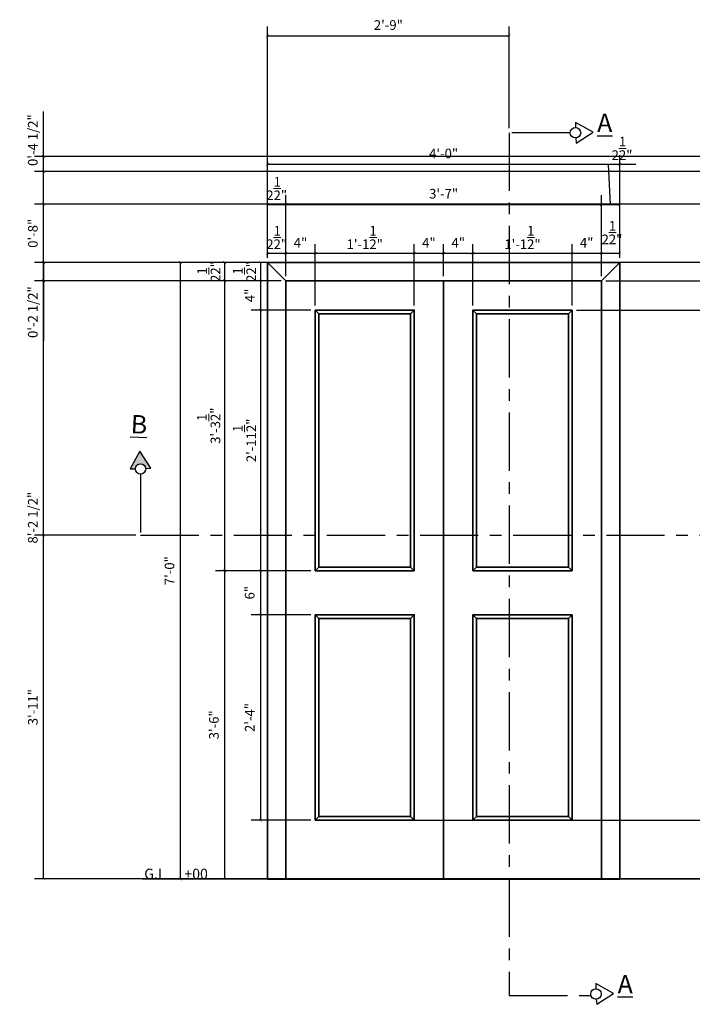
# Model space of a CAD drawing. Units: inches. Extents: x 1926 to 2169, y 1541 to 1783.
# Tile 2 of 3: x 1933 to 2025, y 1649 to 1783. Entities that reach past the tile are written whole.
import ezdxf

# ---------------------------------------------------------------- set-up
doc = ezdxf.new("R2010")
doc.units = ezdxf.units.IN
doc.linetypes.add('CENTER', pattern=[50.8, 31.75, -6.35, 6.35, -6.35])
for name, color, linetype, lineweight in [('A-ANNO-DIMS', 2, 'Continuous', 18), ('A-ANNO-SECT', 1, 'CENTER', 25), ('A-ANNO-SYMB', 1, 'Continuous', 25), ('A-DOOR', 4, 'Continuous', 35)]:
    doc.layers.add(name, color=color, linetype=linetype, lineweight=lineweight)
doc.styles.get("Standard").update_dxf_attribs({"font": 'arial.ttf'})
doc.dimstyles.new('ISO-25', dxfattribs={"dimtxt": 1.3125, "dimasz": 0.375, "dimexe": 1.25, "dimexo": 0.625, "dimtad": 1, "dimzin": 3, "dimlunit": 4, "dimtxsty": 'Standard', "dimblk": 'ARCHTICK', "dimcen": 0.09, "dimadec": 0, "dimazin": 0, "dimtfac": 1, "dimtofl": 0, "dimtmove": 0, "dimatfit": 3, "dimfxl": 1, "dimarcsym": 0})
pattern_1 = [(0, (0, 0), (0, 6.985), [5.08, -1.905]), (90, (0, 0), (-6.985, 4e-16), [5.08, -1.905])]

# ---------------------------------------------------------------- blocks, each defined once
blk = doc.blocks.new('_ArchTick')
at = {"color": 0, "linetype": 'ByBlock', "const_width": 0.15}
blk.add_lwpolyline([(-0.5, -0.5), (0.5, 0.5)], dxfattribs=at)
blk = doc.blocks.new('*D7')
at = {"layer": 'A-ANNO-DIMS', "color": 0, "lineweight": -2, "transparency": 16777216}
for p, q in [((1967.28, 1750.43), (1967.28, 1752.29)), ((1969.78, 1747.93), (1969.78, 1752.29)), ((1967.28, 1751.04), (1969.78, 1751.04))]:
    blk.add_line(p, q, dxfattribs=at)
at = {"layer": 'DEFPOINTS', "color": 0, "transparency": 16777216}
for p in [(1969.78, 1751.04), (1967.28, 1749.81), (1969.78, 1747.31)]:
    blk.add_point(p, dxfattribs=at)
at = {"layer": 'A-ANNO-DIMS', "color": 0, "lineweight": -2, "transparency": 16777216, "xscale": 0.375, "yscale": 0.375, "zscale": 0.375, "rotation": 180}
blk.add_blockref('_ArchTick', (1967.28, 1751.04), dxfattribs=at)
at = {"layer": 'A-ANNO-DIMS', "color": 0, "lineweight": -2, "transparency": 16777216, "xscale": 0.375, "yscale": 0.375, "zscale": 0.375}
blk.add_blockref('_ArchTick', (1969.78, 1751.04), dxfattribs=at)
at = {"layer": 'A-ANNO-DIMS', "color": 0, "transparency": 16777216, "insert": (1968.53, 1753.2), "char_height": 1.3125, "attachment_point": 5}
blk.add_mtext('2{\\H1x;\\S1/2;}"', dxfattribs=at)
blk = doc.blocks.new('*D8')
at = {"layer": 'A-ANNO-DIMS', "color": 0, "lineweight": -2, "transparency": 16777216}
for p, q in [((1969.78, 1747.93), (1969.78, 1752.29)), ((1973.78, 1743.93), (1973.78, 1752.29)), ((1969.78, 1751.04), (1973.78, 1751.04))]:
    blk.add_line(p, q, dxfattribs=at)
at = {"layer": 'DEFPOINTS', "color": 0, "transparency": 16777216}
for p in [(1973.78, 1751.04), (1969.78, 1747.31), (1973.78, 1743.31)]:
    blk.add_point(p, dxfattribs=at)
at = {"layer": 'A-ANNO-DIMS', "color": 0, "lineweight": -2, "transparency": 16777216, "xscale": 0.375, "yscale": 0.375, "zscale": 0.375, "rotation": 180}
blk.add_blockref('_ArchTick', (1969.78, 1751.04), dxfattribs=at)
at = {"layer": 'A-ANNO-DIMS', "color": 0, "lineweight": -2, "transparency": 16777216, "xscale": 0.375, "yscale": 0.375, "zscale": 0.375}
blk.add_blockref('_ArchTick', (1973.78, 1751.04), dxfattribs=at)
at = {"layer": 'A-ANNO-DIMS', "color": 0, "transparency": 16777216, "insert": (1971.78, 1752.32), "char_height": 1.312, "attachment_point": 5}
blk.add_mtext('4"', dxfattribs=at)
blk = doc.blocks.new('*D9')
at = {"layer": 'A-ANNO-DIMS', "color": 0, "lineweight": -2, "transparency": 16777216}
for p, q in [((1973.78, 1743.93), (1973.78, 1752.29)), ((1987.28, 1743.93), (1987.28, 1752.29)), ((1973.78, 1751.04), (1987.28, 1751.04))]:
    blk.add_line(p, q, dxfattribs=at)
at = {"layer": 'DEFPOINTS', "color": 0, "transparency": 16777216}
for p in [(1987.28, 1751.04), (1973.78, 1743.31), (1987.28, 1743.31)]:
    blk.add_point(p, dxfattribs=at)
at = {"layer": 'A-ANNO-DIMS', "color": 0, "lineweight": -2, "transparency": 16777216, "xscale": 0.375, "yscale": 0.375, "zscale": 0.375, "rotation": 180}
blk.add_blockref('_ArchTick', (1973.78, 1751.04), dxfattribs=at)
at = {"layer": 'A-ANNO-DIMS', "color": 0, "lineweight": -2, "transparency": 16777216, "xscale": 0.375, "yscale": 0.375, "zscale": 0.375}
blk.add_blockref('_ArchTick', (1987.28, 1751.04), dxfattribs=at)
at = {"layer": 'A-ANNO-DIMS', "color": 0, "transparency": 16777216, "insert": (1980.53, 1753.2), "char_height": 1.3125, "attachment_point": 5}
blk.add_mtext('1\'-1{\\H1x;\\S1/2;}"', dxfattribs=at)
blk = doc.blocks.new('*D10')
at = {"layer": 'A-ANNO-DIMS', "color": 0, "lineweight": -2, "transparency": 16777216}
for p, q in [((1987.28, 1743.93), (1987.28, 1752.29)), ((1991.28, 1747.93), (1991.28, 1752.29)), ((1987.28, 1751.04), (1991.28, 1751.04))]:
    blk.add_line(p, q, dxfattribs=at)
at = {"layer": 'DEFPOINTS', "color": 0, "transparency": 16777216}
for p in [(1991.28, 1751.04), (1991.28, 1747.31), (1987.28, 1743.31)]:
    blk.add_point(p, dxfattribs=at)
at = {"layer": 'A-ANNO-DIMS', "color": 0, "lineweight": -2, "transparency": 16777216, "xscale": 0.375, "yscale": 0.375, "zscale": 0.375, "rotation": 180}
blk.add_blockref('_ArchTick', (1987.28, 1751.04), dxfattribs=at)
at = {"layer": 'A-ANNO-DIMS', "color": 0, "lineweight": -2, "transparency": 16777216, "xscale": 0.375, "yscale": 0.375, "zscale": 0.375}
blk.add_blockref('_ArchTick', (1991.28, 1751.04), dxfattribs=at)
at = {"layer": 'A-ANNO-DIMS', "color": 0, "transparency": 16777216, "insert": (1989.28, 1752.32), "char_height": 1.312, "attachment_point": 5}
blk.add_mtext('4"', dxfattribs=at)
blk = doc.blocks.new('*D11')
at = {"layer": 'A-ANNO-DIMS', "color": 0, "lineweight": -2, "transparency": 16777216}
for p, q in [((1991.28, 1747.93), (1991.28, 1752.29)), ((1995.28, 1743.93), (1995.28, 1752.29)), ((1991.28, 1751.04), (1995.28, 1751.04))]:
    blk.add_line(p, q, dxfattribs=at)
at = {"layer": 'DEFPOINTS', "color": 0, "transparency": 16777216}
for p in [(1995.28, 1751.04), (1991.28, 1747.31), (1995.28, 1743.31)]:
    blk.add_point(p, dxfattribs=at)
at = {"layer": 'A-ANNO-DIMS', "color": 0, "lineweight": -2, "transparency": 16777216, "xscale": 0.375, "yscale": 0.375, "zscale": 0.375, "rotation": 180}
blk.add_blockref('_ArchTick', (1991.28, 1751.04), dxfattribs=at)
at = {"layer": 'A-ANNO-DIMS', "color": 0, "lineweight": -2, "transparency": 16777216, "xscale": 0.375, "yscale": 0.375, "zscale": 0.375}
blk.add_blockref('_ArchTick', (1995.28, 1751.04), dxfattribs=at)
at = {"layer": 'A-ANNO-DIMS', "color": 0, "transparency": 16777216, "insert": (1993.28, 1752.32), "char_height": 1.312, "attachment_point": 5}
blk.add_mtext('4"', dxfattribs=at)
blk = doc.blocks.new('*D12')
at = {"layer": 'A-ANNO-DIMS', "color": 0, "lineweight": -2, "transparency": 16777216}
for p, q in [((1995.28, 1743.93), (1995.28, 1752.29)), ((2008.78, 1743.93), (2008.78, 1752.29)), ((1995.28, 1751.04), (2008.78, 1751.04))]:
    blk.add_line(p, q, dxfattribs=at)
at = {"layer": 'DEFPOINTS', "color": 0, "transparency": 16777216}
for p in [(2008.78, 1751.04), (1995.28, 1743.31), (2008.78, 1743.31)]:
    blk.add_point(p, dxfattribs=at)
at = {"layer": 'A-ANNO-DIMS', "color": 0, "lineweight": -2, "transparency": 16777216, "xscale": 0.375, "yscale": 0.375, "zscale": 0.375, "rotation": 180}
blk.add_blockref('_ArchTick', (1995.28, 1751.04), dxfattribs=at)
at = {"layer": 'A-ANNO-DIMS', "color": 0, "lineweight": -2, "transparency": 16777216, "xscale": 0.375, "yscale": 0.375, "zscale": 0.375}
blk.add_blockref('_ArchTick', (2008.78, 1751.04), dxfattribs=at)
at = {"layer": 'A-ANNO-DIMS', "color": 0, "transparency": 16777216, "insert": (2002.03, 1753.2), "char_height": 1.3125, "attachment_point": 5}
blk.add_mtext('1\'-1{\\H1x;\\S1/2;}"', dxfattribs=at)
blk = doc.blocks.new('*D13')
at = {"layer": 'A-ANNO-DIMS', "color": 0, "lineweight": -2, "transparency": 16777216}
for p, q in [((2008.78, 1743.93), (2008.78, 1752.29)), ((2012.78, 1747.93), (2012.78, 1752.29)), ((2008.78, 1751.04), (2012.78, 1751.04))]:
    blk.add_line(p, q, dxfattribs=at)
at = {"layer": 'DEFPOINTS', "color": 0, "transparency": 16777216}
for p in [(2012.78, 1751.04), (2012.78, 1747.31), (2008.78, 1743.31)]:
    blk.add_point(p, dxfattribs=at)
at = {"layer": 'A-ANNO-DIMS', "color": 0, "lineweight": -2, "transparency": 16777216, "xscale": 0.375, "yscale": 0.375, "zscale": 0.375, "rotation": 180}
blk.add_blockref('_ArchTick', (2008.78, 1751.04), dxfattribs=at)
at = {"layer": 'A-ANNO-DIMS', "color": 0, "lineweight": -2, "transparency": 16777216, "xscale": 0.375, "yscale": 0.375, "zscale": 0.375}
blk.add_blockref('_ArchTick', (2012.78, 1751.04), dxfattribs=at)
at = {"layer": 'A-ANNO-DIMS', "color": 0, "transparency": 16777216, "insert": (2010.78, 1752.32), "char_height": 1.312, "attachment_point": 5}
blk.add_mtext('4"', dxfattribs=at)
blk = doc.blocks.new('*D14')
at = {"layer": 'A-ANNO-DIMS', "color": 0, "lineweight": -2, "transparency": 16777216}
for p, q in [((2012.78, 1747.93), (2012.78, 1752.29)), ((2015.28, 1750.43), (2015.28, 1752.29)), ((2012.78, 1751.04), (2015.28, 1751.04))]:
    blk.add_line(p, q, dxfattribs=at)
at = {"layer": 'DEFPOINTS', "color": 0, "transparency": 16777216}
for p in [(2015.28, 1751.04), (2015.28, 1749.81), (2012.78, 1747.31)]:
    blk.add_point(p, dxfattribs=at)
at = {"layer": 'A-ANNO-DIMS', "color": 0, "lineweight": -2, "transparency": 16777216, "xscale": 0.375, "yscale": 0.375, "zscale": 0.375, "rotation": 180}
blk.add_blockref('_ArchTick', (2012.78, 1751.04), dxfattribs=at)
at = {"layer": 'A-ANNO-DIMS', "color": 0, "lineweight": -2, "transparency": 16777216, "xscale": 0.375, "yscale": 0.375, "zscale": 0.375}
blk.add_blockref('_ArchTick', (2015.28, 1751.04), dxfattribs=at)
at = {"layer": 'A-ANNO-DIMS', "color": 0, "transparency": 16777216, "insert": (2014.23, 1753.86), "char_height": 1.3125, "attachment_point": 5}
blk.add_mtext('2{\\H1x;\\S1/2;}"', dxfattribs=at)
blk = doc.blocks.new('*D15')
at = {"layer": 'A-ANNO-DIMS', "color": 0, "lineweight": -2, "transparency": 16777216}
for p, q in [((1967.28, 1750.43), (1967.28, 1764.43)), ((2015.28, 1750.43), (2015.28, 1764.43)), ((1967.28, 1763.18), (2015.28, 1763.18))]:
    blk.add_line(p, q, dxfattribs=at)
at = {"layer": 'DEFPOINTS', "color": 0, "transparency": 16777216}
for p in [(2015.28, 1763.18), (1967.28, 1749.81), (2015.28, 1749.81)]:
    blk.add_point(p, dxfattribs=at)
at = {"layer": 'A-ANNO-DIMS', "color": 0, "lineweight": -2, "transparency": 16777216, "xscale": 0.375, "yscale": 0.375, "zscale": 0.375, "rotation": 180}
blk.add_blockref('_ArchTick', (1967.28, 1763.18), dxfattribs=at)
at = {"layer": 'A-ANNO-DIMS', "color": 0, "lineweight": -2, "transparency": 16777216, "xscale": 0.375, "yscale": 0.375, "zscale": 0.375}
blk.add_blockref('_ArchTick', (2015.28, 1763.18), dxfattribs=at)
at = {"layer": 'A-ANNO-DIMS', "color": 0, "transparency": 16777216, "insert": (1991.28, 1764.47), "char_height": 1.312, "attachment_point": 5}
blk.add_mtext('4\'-0"', dxfattribs=at)
blk = doc.blocks.new('*D16')
at = {"layer": 'A-ANNO-DIMS', "color": 0, "lineweight": -2, "transparency": 16777216}
for p, q in [((1967.28, 1750.43), (1967.28, 1758.95)), ((1969.78, 1747.93), (1969.78, 1758.95)), ((1967.28, 1757.7), (1969.78, 1757.7))]:
    blk.add_line(p, q, dxfattribs=at)
at = {"layer": 'DEFPOINTS', "color": 0, "transparency": 16777216}
for p in [(1969.78, 1757.7), (1967.28, 1749.81), (1969.78, 1747.31)]:
    blk.add_point(p, dxfattribs=at)
at = {"layer": 'A-ANNO-DIMS', "color": 0, "lineweight": -2, "transparency": 16777216, "xscale": 0.375, "yscale": 0.375, "zscale": 0.375, "rotation": 180}
blk.add_blockref('_ArchTick', (1967.28, 1757.7), dxfattribs=at)
at = {"layer": 'A-ANNO-DIMS', "color": 0, "lineweight": -2, "transparency": 16777216, "xscale": 0.375, "yscale": 0.375, "zscale": 0.375}
blk.add_blockref('_ArchTick', (1969.78, 1757.7), dxfattribs=at)
at = {"layer": 'A-ANNO-DIMS', "color": 0, "transparency": 16777216, "insert": (1968.53, 1759.86), "char_height": 1.3125, "attachment_point": 5}
blk.add_mtext('2{\\H1x;\\S1/2;}"', dxfattribs=at)
blk = doc.blocks.new('*D17')
at = {"layer": 'A-ANNO-DIMS', "color": 0, "lineweight": -2, "transparency": 16777216}
for p, q in [((1969.78, 1747.93), (1969.78, 1758.95)), ((2012.78, 1747.93), (2012.78, 1758.95)), ((1969.78, 1757.7), (2012.78, 1757.7))]:
    blk.add_line(p, q, dxfattribs=at)
at = {"layer": 'DEFPOINTS', "color": 0, "transparency": 16777216}
for p in [(2012.78, 1757.7), (1969.78, 1747.31), (2012.78, 1747.31)]:
    blk.add_point(p, dxfattribs=at)
at = {"layer": 'A-ANNO-DIMS', "color": 0, "lineweight": -2, "transparency": 16777216, "xscale": 0.375, "yscale": 0.375, "zscale": 0.375, "rotation": 180}
blk.add_blockref('_ArchTick', (1969.78, 1757.7), dxfattribs=at)
at = {"layer": 'A-ANNO-DIMS', "color": 0, "lineweight": -2, "transparency": 16777216, "xscale": 0.375, "yscale": 0.375, "zscale": 0.375}
blk.add_blockref('_ArchTick', (2012.78, 1757.7), dxfattribs=at)
at = {"layer": 'A-ANNO-DIMS', "color": 0, "transparency": 16777216, "insert": (1991.28, 1758.99), "char_height": 1.312, "attachment_point": 5}
blk.add_mtext('3\'-7"', dxfattribs=at)
blk = doc.blocks.new('*D18')
at = {"layer": 'A-ANNO-DIMS', "color": 0, "lineweight": -2, "transparency": 16777216}
for p, q in [((2014.03, 1757.7), (2013.74, 1763.18)), ((2013.74, 1763.18), (2017.47, 1763.18)), ((2012.78, 1747.93), (2012.78, 1758.95)), ((2015.28, 1750.43), (2015.28, 1758.95)), ((2012.78, 1757.7), (2015.28, 1757.7))]:
    blk.add_line(p, q, dxfattribs=at)
at = {"layer": 'DEFPOINTS', "color": 0, "transparency": 16777216}
for p in [(2015.28, 1757.7), (2015.28, 1749.81), (2012.78, 1747.31)]:
    blk.add_point(p, dxfattribs=at)
at = {"layer": 'A-ANNO-DIMS', "color": 0, "lineweight": -2, "transparency": 16777216, "xscale": 0.375, "yscale": 0.375, "zscale": 0.375, "rotation": 180}
blk.add_blockref('_ArchTick', (2012.78, 1757.7), dxfattribs=at)
at = {"layer": 'A-ANNO-DIMS', "color": 0, "lineweight": -2, "transparency": 16777216, "xscale": 0.375, "yscale": 0.375, "zscale": 0.375}
blk.add_blockref('_ArchTick', (2015.28, 1757.7), dxfattribs=at)
at = {"layer": 'A-ANNO-DIMS', "color": 0, "transparency": 16777216, "insert": (2015.6, 1765.34), "char_height": 1.3125, "attachment_point": 5}
blk.add_mtext('2{\\H1x;\\S1/2;}"', dxfattribs=at)
blk = doc.blocks.new('*D19')
at = {"layer": 'A-ANNO-DIMS', "color": 0, "lineweight": -2, "transparency": 16777216}
for p, q in [((1966.66, 1749.81), (1965.05, 1749.81)), ((1966.3, 1749.81), (1966.3, 1747.31)), ((1969.16, 1747.31), (1965.05, 1747.31))]:
    blk.add_line(p, q, dxfattribs=at)
at = {"layer": 'DEFPOINTS', "color": 0, "transparency": 16777216}
for p in [(1967.28, 1749.81), (1966.3, 1747.31), (1969.78, 1747.31)]:
    blk.add_point(p, dxfattribs=at)
at = {"layer": 'A-ANNO-DIMS', "color": 0, "lineweight": -2, "transparency": 16777216, "xscale": 0.375, "yscale": 0.375, "zscale": 0.375}
for p, rotation in [((1966.3, 1749.81), 90), ((1966.3, 1747.31), 270)]:
    blk.add_blockref('_ArchTick', p, dxfattribs=dict(at, rotation=rotation))
at = {"layer": 'A-ANNO-DIMS', "color": 0, "transparency": 16777216, "insert": (1964.14, 1748.56), "char_height": 1.3125, "attachment_point": 5, "rotation": 90}
blk.add_mtext('2{\\H1x;\\S1/2;}"', dxfattribs=at)
blk = doc.blocks.new('*D20')
at = {"layer": 'A-ANNO-DIMS', "color": 0, "lineweight": -2, "transparency": 16777216}
for p, q in [((1969.16, 1747.31), (1965.05, 1747.31)), ((1966.3, 1747.31), (1966.3, 1743.31)), ((1973.16, 1743.31), (1965.05, 1743.31))]:
    blk.add_line(p, q, dxfattribs=at)
at = {"layer": 'DEFPOINTS', "color": 0, "transparency": 16777216}
for p in [(1969.78, 1747.31), (1966.3, 1743.31), (1973.78, 1743.31)]:
    blk.add_point(p, dxfattribs=at)
at = {"layer": 'A-ANNO-DIMS', "color": 0, "lineweight": -2, "transparency": 16777216, "xscale": 0.375, "yscale": 0.375, "zscale": 0.375}
for p, rotation in [((1966.3, 1747.31), 90), ((1966.3, 1743.31), 270)]:
    blk.add_blockref('_ArchTick', p, dxfattribs=dict(at, rotation=rotation))
at = {"layer": 'A-ANNO-DIMS', "color": 0, "transparency": 16777216, "insert": (1965.02, 1745.31), "char_height": 1.312, "attachment_point": 5, "rotation": 90}
blk.add_mtext('4"', dxfattribs=at)
blk = doc.blocks.new('*D21')
at = {"layer": 'A-ANNO-DIMS', "color": 0, "lineweight": -2, "transparency": 16777216}
for p, q in [((1973.16, 1743.31), (1965.05, 1743.31)), ((1966.3, 1743.31), (1966.3, 1707.81)), ((1973.16, 1707.81), (1965.05, 1707.81))]:
    blk.add_line(p, q, dxfattribs=at)
at = {"layer": 'DEFPOINTS', "color": 0, "transparency": 16777216}
for p in [(1973.78, 1743.31), (1966.3, 1707.81), (1973.78, 1707.81)]:
    blk.add_point(p, dxfattribs=at)
at = {"layer": 'A-ANNO-DIMS', "color": 0, "lineweight": -2, "transparency": 16777216, "xscale": 0.375, "yscale": 0.375, "zscale": 0.375}
for p, rotation in [((1966.3, 1743.31), 90), ((1966.3, 1707.81), 270)]:
    blk.add_blockref('_ArchTick', p, dxfattribs=dict(at, rotation=rotation))
at = {"layer": 'A-ANNO-DIMS', "color": 0, "transparency": 16777216, "insert": (1964.14, 1725.56), "char_height": 1.3125, "attachment_point": 5, "rotation": 90}
blk.add_mtext('2\'-11{\\H1x;\\S1/2;}"', dxfattribs=at)
blk = doc.blocks.new('*D22')
at = {"layer": 'A-ANNO-DIMS', "color": 0, "lineweight": -2, "transparency": 16777216}
for p, q in [((1973.16, 1707.81), (1965.05, 1707.81)), ((1966.3, 1707.81), (1966.3, 1701.81)), ((1973.16, 1701.81), (1965.05, 1701.81))]:
    blk.add_line(p, q, dxfattribs=at)
at = {"layer": 'DEFPOINTS', "color": 0, "transparency": 16777216}
for p in [(1973.78, 1707.81), (1966.3, 1701.81), (1973.78, 1701.81)]:
    blk.add_point(p, dxfattribs=at)
at = {"layer": 'A-ANNO-DIMS', "color": 0, "lineweight": -2, "transparency": 16777216, "xscale": 0.375, "yscale": 0.375, "zscale": 0.375}
for p, rotation in [((1966.3, 1707.81), 90), ((1966.3, 1701.81), 270)]:
    blk.add_blockref('_ArchTick', p, dxfattribs=dict(at, rotation=rotation))
at = {"layer": 'A-ANNO-DIMS', "color": 0, "transparency": 16777216, "insert": (1965.01, 1704.81), "char_height": 1.312, "attachment_point": 5, "rotation": 90}
blk.add_mtext('6"', dxfattribs=at)
blk = doc.blocks.new('*D23')
at = {"layer": 'A-ANNO-DIMS', "color": 0, "lineweight": -2, "transparency": 16777216}
for p, q in [((1973.16, 1701.81), (1965.05, 1701.81)), ((1966.3, 1701.81), (1966.3, 1673.81)), ((1973.16, 1673.81), (1965.05, 1673.81))]:
    blk.add_line(p, q, dxfattribs=at)
at = {"layer": 'DEFPOINTS', "color": 0, "transparency": 16777216}
for p in [(1973.78, 1701.81), (1966.3, 1673.81), (1973.78, 1673.81)]:
    blk.add_point(p, dxfattribs=at)
at = {"layer": 'A-ANNO-DIMS', "color": 0, "lineweight": -2, "transparency": 16777216, "xscale": 0.375, "yscale": 0.375, "zscale": 0.375}
for p, rotation in [((1966.3, 1701.81), 90), ((1966.3, 1673.81), 270)]:
    blk.add_blockref('_ArchTick', p, dxfattribs=dict(at, rotation=rotation))
at = {"layer": 'A-ANNO-DIMS', "color": 0, "transparency": 16777216, "insert": (1965.02, 1687.81), "char_height": 1.312, "attachment_point": 5, "rotation": 90}
blk.add_mtext('2\'-4"', dxfattribs=at)
blk = doc.blocks.new('*D24')
at = {"layer": 'A-ANNO-DIMS', "color": 0, "lineweight": -2, "transparency": 16777216}
for p, q in [((1974.41, 1673.81), (2129.74, 1673.81)), ((2128.49, 1673.81), (2128.49, 1665.81)), ((2134.77, 1665.81), (2127.24, 1665.81))]:
    blk.add_line(p, q, dxfattribs=at)
at = {"layer": 'DEFPOINTS', "color": 0, "transparency": 16777216}
for p in [(1973.78, 1673.81), (2128.49, 1665.81), (2135.4, 1665.81)]:
    blk.add_point(p, dxfattribs=at)
at = {"layer": 'A-ANNO-DIMS', "color": 0, "lineweight": -2, "transparency": 16777216, "xscale": 0.375, "yscale": 0.375, "zscale": 0.375}
for p, rotation in [((2128.49, 1673.81), 90), ((2128.49, 1665.81), 270)]:
    blk.add_blockref('_ArchTick', p, dxfattribs=dict(at, rotation=rotation))
at = {"layer": 'A-ANNO-DIMS', "color": 0, "transparency": 16777216, "insert": (2127.2, 1669.81), "char_height": 1.312, "attachment_point": 5, "rotation": 90}
blk.add_mtext('8"', dxfattribs=at)
blk = doc.blocks.new('*D25')
at = {"layer": 'A-ANNO-DIMS', "color": 0, "lineweight": -2, "transparency": 16777216}
for p, q in [((1966.66, 1749.81), (1960.18, 1749.81)), ((1961.43, 1749.81), (1961.43, 1747.31)), ((1969.16, 1747.31), (1960.18, 1747.31))]:
    blk.add_line(p, q, dxfattribs=at)
at = {"layer": 'DEFPOINTS', "color": 0, "transparency": 16777216}
for p in [(1967.28, 1749.81), (1961.43, 1747.31), (1969.78, 1747.31)]:
    blk.add_point(p, dxfattribs=at)
at = {"layer": 'A-ANNO-DIMS', "color": 0, "lineweight": -2, "transparency": 16777216, "xscale": 0.375, "yscale": 0.375, "zscale": 0.375}
for p, rotation in [((1961.43, 1749.81), 90), ((1961.43, 1747.31), 270)]:
    blk.add_blockref('_ArchTick', p, dxfattribs=dict(at, rotation=rotation))
at = {"layer": 'A-ANNO-DIMS', "color": 0, "transparency": 16777216, "insert": (1959.27, 1748.56), "char_height": 1.3125, "attachment_point": 5, "rotation": 90}
blk.add_mtext('2{\\H1x;\\S1/2;}"', dxfattribs=at)
blk = doc.blocks.new('*D26')
at = {"layer": 'A-ANNO-DIMS', "color": 0, "lineweight": -2, "transparency": 16777216}
for p, q in [((1969.16, 1747.31), (1960.18, 1747.31)), ((1961.43, 1747.31), (1961.43, 1707.81)), ((1973.16, 1707.81), (1960.18, 1707.81))]:
    blk.add_line(p, q, dxfattribs=at)
at = {"layer": 'DEFPOINTS', "color": 0, "transparency": 16777216}
for p in [(1969.78, 1747.31), (1961.43, 1707.81), (1973.78, 1707.81)]:
    blk.add_point(p, dxfattribs=at)
at = {"layer": 'A-ANNO-DIMS', "color": 0, "lineweight": -2, "transparency": 16777216, "xscale": 0.375, "yscale": 0.375, "zscale": 0.375}
for p, rotation in [((1961.43, 1747.31), 90), ((1961.43, 1707.81), 270)]:
    blk.add_blockref('_ArchTick', p, dxfattribs=dict(at, rotation=rotation))
at = {"layer": 'A-ANNO-DIMS', "color": 0, "transparency": 16777216, "insert": (1959.26, 1727.56), "char_height": 1.3125, "attachment_point": 5, "rotation": 90}
blk.add_mtext('3\'-3{\\H1x;\\S1/2;}"', dxfattribs=at)
blk = doc.blocks.new('*D27')
at = {"layer": 'A-ANNO-DIMS', "color": 0, "lineweight": -2, "transparency": 16777216}
for p, q in [((1973.16, 1707.81), (1960.18, 1707.81)), ((1961.43, 1707.81), (1961.43, 1665.81)), ((1969.16, 1665.81), (1960.18, 1665.81))]:
    blk.add_line(p, q, dxfattribs=at)
at = {"layer": 'DEFPOINTS', "color": 0, "transparency": 16777216}
for p in [(1973.78, 1707.81), (1961.43, 1665.81), (1969.78, 1665.81)]:
    blk.add_point(p, dxfattribs=at)
at = {"layer": 'A-ANNO-DIMS', "color": 0, "lineweight": -2, "transparency": 16777216, "xscale": 0.375, "yscale": 0.375, "zscale": 0.375}
for p, rotation in [((1961.43, 1707.81), 90), ((1961.43, 1665.81), 270)]:
    blk.add_blockref('_ArchTick', p, dxfattribs=dict(at, rotation=rotation))
at = {"layer": 'A-ANNO-DIMS', "color": 0, "transparency": 16777216, "insert": (1960.14, 1686.81), "char_height": 1.312, "attachment_point": 5, "rotation": 90}
blk.add_mtext('3\'-6"', dxfattribs=at)
blk = doc.blocks.new('*D28')
at = {"layer": 'A-ANNO-DIMS', "color": 0, "lineweight": -2, "transparency": 16777216}
for p, q in [((1966.66, 1749.81), (1954.13, 1749.81)), ((1955.38, 1749.81), (1955.38, 1665.81)), ((2140.71, 1665.81), (1954.13, 1665.81))]:
    blk.add_line(p, q, dxfattribs=at)
at = {"layer": 'DEFPOINTS', "color": 0, "transparency": 16777216}
for p in [(1967.28, 1749.81), (1955.38, 1665.81), (2141.33, 1665.81)]:
    blk.add_point(p, dxfattribs=at)
at = {"layer": 'A-ANNO-DIMS', "color": 0, "lineweight": -2, "transparency": 16777216, "xscale": 0.375, "yscale": 0.375, "zscale": 0.375}
for p, rotation in [((1955.38, 1749.81), 90), ((1955.38, 1665.81), 270)]:
    blk.add_blockref('_ArchTick', p, dxfattribs=dict(at, rotation=rotation))
at = {"layer": 'A-ANNO-DIMS', "color": 0, "transparency": 16777216, "insert": (1954.09, 1707.81), "char_height": 1.312, "attachment_point": 5, "rotation": 90}
blk.add_mtext('7\'-0"', dxfattribs=at)
blk = doc.blocks.new('DOOR-PANEL-UPPER')
for p, q in [((0.5, 35), (0, 35.5)), ((13, 35), (13.5, 35.5)), ((0.5, 0.5), (0, 0)), ((13, 0.5), (13.5, 0))]:
    blk.add_line(p, q)
for points in [[(0, 35.5), (13.5, 35.5), (13.5, 0), (0, 0)], [(0.5, 35), (13, 35), (13, 0.5), (0.5, 0.5)]]:
    blk.add_lwpolyline(points, close=True)
blk = doc.blocks.new('DOOR-PANEL-LOWER')
for p, q in [((0, 28), (0.5, 27.5)), ((13, 27.5), (13.5, 28)), ((0.5, 0.5), (0, 0)), ((13, 0.5), (13.5, 0))]:
    blk.add_line(p, q)
for points in [[(0, 28), (13.5, 28), (13.5, 0), (0, 0)], [(0.5, 27.5), (13, 27.5), (13, 0.5), (0.5, 0.5)]]:
    blk.add_lwpolyline(points, close=True)
blk = doc.blocks.new('*D31')
at = {"layer": 'A-ANNO-DIMS', "color": 0, "lineweight": -2, "transparency": 16777216}
for p, q in [((1966.66, 1749.81), (1935.51, 1749.81)), ((1936.76, 1749.81), (1936.76, 1747.31)), ((1969.16, 1747.31), (1935.51, 1747.31)), ((1936.76, 1747.31), (1936.76, 1739.13))]:
    blk.add_line(p, q, dxfattribs=at)
at = {"layer": 'DEFPOINTS', "color": 0, "transparency": 16777216}
for p in [(1967.28, 1749.81), (1936.76, 1747.31), (1969.78, 1747.31)]:
    blk.add_point(p, dxfattribs=at)
at = {"layer": 'A-ANNO-DIMS', "color": 0, "lineweight": -2, "transparency": 16777216, "xscale": 0.375, "yscale": 0.375, "zscale": 0.375}
for p, rotation in [((1936.76, 1749.81), 90), ((1936.76, 1747.31), 270)]:
    blk.add_blockref('_ArchTick', p, dxfattribs=dict(at, rotation=rotation))
at = {"layer": 'A-ANNO-DIMS', "color": 0, "transparency": 16777216, "insert": (1935.45, 1743.03), "char_height": 1.312, "attachment_point": 5, "rotation": 90}
blk.add_mtext('0\'-2 1/2"', dxfattribs=at)
blk = doc.blocks.new('*D32')
at = {"layer": 'A-ANNO-DIMS', "color": 0, "lineweight": -2, "transparency": 16777216}
for p, q in [((2013.41, 1747.31), (2106.38, 1747.31)), ((2105.13, 1747.31), (2105.13, 1743.31)), ((2009.41, 1743.31), (2106.38, 1743.31)), ((2105.13, 1743.31), (2105.13, 1738.19))]:
    blk.add_line(p, q, dxfattribs=at)
at = {"layer": 'DEFPOINTS', "color": 0, "transparency": 16777216}
for p in [(2012.78, 1747.31), (2008.78, 1743.31), (2105.13, 1743.31)]:
    blk.add_point(p, dxfattribs=at)
at = {"layer": 'A-ANNO-DIMS', "color": 0, "lineweight": -2, "transparency": 16777216, "xscale": 0.375, "yscale": 0.375, "zscale": 0.375}
for p, rotation in [((2105.13, 1747.31), 90), ((2105.13, 1743.31), 270)]:
    blk.add_blockref('_ArchTick', p, dxfattribs=dict(at, rotation=rotation))
at = {"layer": 'A-ANNO-DIMS', "color": 0, "transparency": 16777216, "insert": (2103.84, 1740.56), "char_height": 1.312, "attachment_point": 5, "rotation": 90}
blk.add_mtext('0\'-4"', dxfattribs=at)
blk = doc.blocks.new('*D33')
at = {"layer": 'A-ANNO-DIMS', "color": 0, "lineweight": -2, "transparency": 16777216}
for p, q in [((1967.28, 1750.43), (1967.28, 1781.93)), ((2000.22, 1768.09), (2000.22, 1781.93)), ((1967.28, 1780.68), (2000.22, 1780.68))]:
    blk.add_line(p, q, dxfattribs=at)
at = {"layer": 'DEFPOINTS', "color": 0, "transparency": 16777216}
for p in [(2000.22, 1780.68), (2000.22, 1767.47), (1967.28, 1749.81)]:
    blk.add_point(p, dxfattribs=at)
at = {"layer": 'A-ANNO-DIMS', "color": 0, "lineweight": -2, "transparency": 16777216, "xscale": 0.375, "yscale": 0.375, "zscale": 0.375, "rotation": 180}
blk.add_blockref('_ArchTick', (1967.28, 1780.68), dxfattribs=at)
at = {"layer": 'A-ANNO-DIMS', "color": 0, "lineweight": -2, "transparency": 16777216, "xscale": 0.375, "yscale": 0.375, "zscale": 0.375}
blk.add_blockref('_ArchTick', (2000.22, 1780.68), dxfattribs=at)
at = {"layer": 'A-ANNO-DIMS', "color": 0, "transparency": 16777216, "insert": (1983.75, 1781.97), "char_height": 1.312, "attachment_point": 5}
blk.add_mtext('2\'-9"', dxfattribs=at)
blk = doc.blocks.new('*D34')
at = {"layer": 'A-ANNO-DIMS', "color": 0, "lineweight": -2, "transparency": 16777216}
for p, q in [((1949.34, 1712.64), (1935.51, 1712.64)), ((1936.76, 1665.81), (1936.76, 1712.64)), ((1966.66, 1665.81), (1935.51, 1665.81))]:
    blk.add_line(p, q, dxfattribs=at)
at = {"layer": 'DEFPOINTS', "color": 0, "transparency": 16777216}
for p in [(1936.76, 1712.64), (1949.97, 1712.64), (1967.28, 1665.81)]:
    blk.add_point(p, dxfattribs=at)
at = {"layer": 'A-ANNO-DIMS', "color": 0, "lineweight": -2, "transparency": 16777216, "xscale": 0.375, "yscale": 0.375, "zscale": 0.375}
for p, rotation in [((1936.76, 1712.64), 90), ((1936.76, 1665.81), 270)]:
    blk.add_blockref('_ArchTick', p, dxfattribs=dict(at, rotation=rotation))
at = {"layer": 'A-ANNO-DIMS', "color": 0, "transparency": 16777216, "insert": (1935.46, 1689.22), "char_height": 1.312, "attachment_point": 5, "rotation": 90}
blk.add_mtext('3\'-11"', dxfattribs=at)
blk = doc.blocks.new('*D35')
at = {"layer": 'A-ANNO-DIMS', "color": 0, "lineweight": -2, "transparency": 16777216}
for p, q in [((2054.17, 1764.25), (1935.51, 1764.25)), ((1936.76, 1665.81), (1936.76, 1764.25)), ((2048.92, 1665.81), (1935.51, 1665.81))]:
    blk.add_line(p, q, dxfattribs=at)
at = {"layer": 'DEFPOINTS', "color": 0, "transparency": 16777216}
for p in [(1936.76, 1764.25), (2054.79, 1764.25), (2049.54, 1665.81)]:
    blk.add_point(p, dxfattribs=at)
at = {"layer": 'A-ANNO-DIMS', "color": 0, "lineweight": -2, "transparency": 16777216, "xscale": 0.375, "yscale": 0.375, "zscale": 0.375}
for p, rotation in [((1936.76, 1764.25), 90), ((1936.76, 1665.81), 270)]:
    blk.add_blockref('_ArchTick', p, dxfattribs=dict(at, rotation=rotation))
at = {"layer": 'A-ANNO-DIMS', "color": 0, "transparency": 16777216, "insert": (1935.45, 1715.03), "char_height": 1.312, "attachment_point": 5, "rotation": 90}
blk.add_mtext('8\'-2 1/2"', dxfattribs=at)
blk = doc.blocks.new('*D37')
at = {"layer": 'A-ANNO-DIMS', "color": 0, "lineweight": -2, "transparency": 16777216}
for p, q in [((2048.92, 1757.73), (1935.51, 1757.73)), ((1936.76, 1749.81), (1936.76, 1757.73)), ((2048.92, 1749.81), (1935.51, 1749.81))]:
    blk.add_line(p, q, dxfattribs=at)
at = {"layer": 'DEFPOINTS', "color": 0, "transparency": 16777216}
for p in [(1936.76, 1757.73), (2049.54, 1757.73), (2049.54, 1749.81)]:
    blk.add_point(p, dxfattribs=at)
at = {"layer": 'A-ANNO-DIMS', "color": 0, "lineweight": -2, "transparency": 16777216, "xscale": 0.375, "yscale": 0.375, "zscale": 0.375}
for p, rotation in [((1936.76, 1757.73), 90), ((1936.76, 1749.81), 270)]:
    blk.add_blockref('_ArchTick', p, dxfattribs=dict(at, rotation=rotation))
at = {"layer": 'A-ANNO-DIMS', "color": 0, "transparency": 16777216, "insert": (1935.46, 1753.77), "char_height": 1.312, "attachment_point": 5, "rotation": 90}
blk.add_mtext('0\'-8"', dxfattribs=at)
blk = doc.blocks.new('*D38')
at = {"layer": 'A-ANNO-DIMS', "color": 0, "lineweight": -2, "transparency": 16777216}
for p, q in [((1936.76, 1762.19), (1936.76, 1770.36)), ((2048.92, 1762.19), (1935.51, 1762.19)), ((1936.76, 1757.73), (1936.76, 1762.19)), ((2048.92, 1757.73), (1935.51, 1757.73))]:
    blk.add_line(p, q, dxfattribs=at)
at = {"layer": 'DEFPOINTS', "color": 0, "transparency": 16777216}
for p in [(1936.76, 1762.19), (2049.54, 1762.19), (2049.54, 1757.73)]:
    blk.add_point(p, dxfattribs=at)
at = {"layer": 'A-ANNO-DIMS', "color": 0, "lineweight": -2, "transparency": 16777216, "xscale": 0.375, "yscale": 0.375, "zscale": 0.375}
for p, rotation in [((1936.76, 1762.19), 90), ((1936.76, 1757.73), 270)]:
    blk.add_blockref('_ArchTick', p, dxfattribs=dict(at, rotation=rotation))
at = {"layer": 'A-ANNO-DIMS', "color": 0, "transparency": 16777216, "insert": (1935.45, 1766.46), "char_height": 1.312, "attachment_point": 5, "rotation": 90}
blk.add_mtext('0\'-4 1/2"', dxfattribs=at)

msp = doc.modelspace()

# ---------------------------------------------------------------- hatches: boundary and pattern name
at = {"layer": 'A-ANNO-SYMB'}
h = msp.add_hatch(dxfattribs=at)
h.set_pattern_fill('ANGLE', color=256)
h.set_pattern_definition(pattern_1)
h.paths.add_polyline_path([(2009.25, 1768.878), (2009.25, 1768.182, -0.4142136), (2009.963, 1767.469, -0.3926966), (2009.303, 1766.758), (2009.354, 1766.064), (2011.66, 1767.558)])
h = msp.add_hatch(color=256, dxfattribs=at)
h.dxf.hatch_style = 1
h.paths.add_polyline_path([(1949.877, 1724.078), (1948.557, 1721.669), (1949.253, 1721.669, -0.9636592), (1950.677, 1721.721), (1951.372, 1721.773)])
h = msp.add_hatch(dxfattribs=at)
h.set_pattern_fill('ANGLE', color=256, angle=90)
h.set_pattern_definition([(90, (3705.052, -295.39), (-6.985, 4e-16), [5.08, -1.905]), (180, (3705.052, -295.39), (-9e-16, -6.985), [5.08, -1.905])])
h.paths.add_polyline_path([(1936.174, 1713.86), (1936.87, 1713.86, -0.4142136), (1937.583, 1714.573, -0.3926966), (1938.294, 1713.913), (1938.988, 1713.965), (1937.494, 1716.27)])
h = msp.add_hatch(dxfattribs=at)
h.set_pattern_fill('ANGLE', color=256)
h.set_pattern_definition([(0, (2.793, -117.327), (0, 6.985), [5.08, -1.905]), (90, (2.793, -117.327), (-6.985, 4e-16), [5.08, -1.905])])
h.paths.add_polyline_path([(2012.043, 1651.551), (2012.043, 1650.855, -0.4142136), (2012.756, 1650.142, -0.3926966), (2012.096, 1649.431), (2012.147, 1648.737), (2014.452, 1650.231)])
h = msp.add_hatch(dxfattribs=at)
h.set_pattern_fill('ANGLE', color=256)
h.set_pattern_definition(pattern_1)
h.paths.add_polyline_path([(2014.452, 1650.231), (2012.043, 1651.551), (2012.043, 1650.855, -0.4142136), (2012.756, 1650.142, -0.3926966), (2012.096, 1649.431), (2012.147, 1648.737)])

# ---------------------------------------------------------------- linework, layer by layer
at = {"layer": 'A-ANNO-SECT', "ltscale": 0.25}
for points in [[(2008.537, 1767.469), (2000.221, 1767.469), (2000.221, 1649.925), (2011.364, 1649.925)], [(1949.966, 1720.956), (1949.966, 1712.639), (2030.915, 1712.639), (2030.915, 1723.782)]]:
    msp.add_lwpolyline(points, dxfattribs=at)
at = {"layer": 'A-ANNO-SYMB'}
msp.add_line((2093.331, 1665.806), (1950.218, 1665.806), dxfattribs=at)
for points in [[(2009.303, 1766.758), (2009.354, 1766.064), (2011.66, 1767.558), (2009.25, 1768.878), (2009.25, 1768.182)], [(1950.677, 1721.721), (1951.372, 1721.773), (1949.877, 1724.078), (1948.557, 1721.669), (1949.253, 1721.669)], [(2012.096, 1649.431), (2012.147, 1648.737), (2014.452, 1650.231), (2012.043, 1651.551), (2012.043, 1650.855)]]:
    msp.add_lwpolyline(points, dxfattribs=at)
for centre in [(2009.25, 1767.469), (1949.966, 1721.669), (2012.043, 1650.142)]:
    msp.add_circle(centre, 0.713, dxfattribs=at)
at = {"layer": 'A-DOOR'}
for p, q in [((1969.78, 1747.306), (1967.28, 1749.806)), ((2012.78, 1747.306), (2015.28, 1749.806)), ((1991.28, 1747.306), (1991.28, 1665.806))]:
    msp.add_line(p, q, dxfattribs=at)
msp.add_lwpolyline([(1967.28, 1749.806), (2015.28, 1749.806), (2015.28, 1665.806), (1967.28, 1665.806)], close=True, dxfattribs=at)
msp.add_lwpolyline([(1969.78, 1665.806), (1969.78, 1747.306), (2012.78, 1747.306), (2012.78, 1665.806)], dxfattribs=at)

# ---------------------------------------------------------------- block references
for name, p in [('DOOR-PANEL-UPPER', (1973.78, 1707.806)), ('DOOR-PANEL-LOWER', (1973.78, 1673.806))]:
    msp.add_blockref(name, p, dxfattribs=at)
at = {"layer": 'A-DOOR', "extrusion": (0, 0, -1), "zscale": -1}
for name, p in [('DOOR-PANEL-UPPER', (-2008.781, 1707.806)), ('DOOR-PANEL-LOWER', (-2008.781, 1673.806))]:
    msp.add_blockref(name, p, dxfattribs=at)

# ---------------------------------------------------------------- texts
at = {"layer": 'A-ANNO-SYMB'}
msp.add_text('G.L      +00', height=1.40571, dxfattribs=at).set_placement((1950.477, 1665.806))
at = {"layer": 'A-ANNO-SYMB', "char_height": 2.5, "attachment_point": 1}
for insert in [(2012.205, 1770.068), (2014.998, 1652.741)]:
    msp.add_mtext_dynamic_manual_height_columns('{\\LA}', width=4.12722, gutter_width=12.5, heights=[0], dxfattribs=dict(at, insert=insert))
at = {"layer": 'A-ANNO-SYMB', "insert": (1948.699, 1729.043), "char_height": 2.5, "attachment_point": 1, "rotation": 357.55115}
msp.add_mtext_dynamic_manual_height_columns('{\\LB}', width=4.12722, gutter_width=12.5, heights=[0], dxfattribs=at)

# ---------------------------------------------------------------- dimensions: what is measured, and where the dimension line sits
at = {"layer": 'A-ANNO-DIMS'}
for base, p1, p2, override, picture, middle in [((2000.221, 1780.678), (1967.28, 1749.806), (2000.221, 1767.469), {"dimdec": 1, "dimlfac": 1, "dimrnd": 0, "dimzin": 1, "dimdsep": 46, "dimlunit": 4, "dimfrac": 2}, '*D33', (1983.751, 1781.974)), ((2015.28, 1763.178), (1967.28, 1749.806), (2015.28, 1749.806), {"dimclrd": 0, "dimclre": 0, "dimclrt": 0}, '*D15', (1991.28, 1764.473)), ((2012.78, 1757.698), (1969.78, 1747.306), (2012.78, 1747.306), {"dimclrd": 0, "dimclre": 0, "dimclrt": 0, "dimtmove": 1}, '*D17', (1991.28, 1758.994)), ((1987.28, 1751.038), (1973.78, 1743.306), (1987.28, 1743.306), {"dimclrd": 0, "dimclre": 0, "dimclrt": 0, "dimtmove": 1}, '*D9', (1980.53, 1753.2)), ((2008.78, 1751.038), (1995.28, 1743.306), (2008.78, 1743.306), {"dimclrd": 0, "dimclre": 0, "dimclrt": 0, "dimtmove": 1}, '*D12', (2002.03, 1753.2)), ((1973.78, 1751.038), (1969.78, 1747.306), (1973.78, 1743.306), {"dimclrd": 0, "dimclre": 0, "dimclrt": 0, "dimtmove": 1}, '*D8', (1971.78, 1752.32)), ((1991.28, 1751.038), (1987.28, 1743.306), (1991.28, 1747.306), {"dimclrd": 0, "dimclre": 0, "dimclrt": 0, "dimtmove": 1}, '*D10', (1989.28, 1752.32)), ((1995.28, 1751.038), (1991.28, 1747.306), (1995.28, 1743.306), {"dimclrd": 0, "dimclre": 0, "dimclrt": 0, "dimtmove": 1}, '*D11', (1993.28, 1752.32)), ((2012.78, 1751.038), (2008.78, 1743.306), (2012.78, 1747.306), {"dimclrd": 0, "dimclre": 0, "dimclrt": 0, "dimtmove": 1}, '*D13', (2010.78, 1752.32))]:
    dim = msp.add_linear_dim(base=base, p1=p1, p2=p2, dimstyle='ISO-25', override=override, dxfattribs=at)
    dim.commit()
    dim.dimension.update_dxf_attribs({"geometry": picture, "text_midpoint": middle})
for base, p1, p2, override, picture, middle in [((1936.757, 1762.19), (2049.54, 1757.726), (2049.54, 1762.19), {"dimdec": 1, "dimlfac": 1, "dimrnd": 0, "dimzin": 1, "dimdsep": 46, "dimlunit": 4, "dimfrac": 2}, '*D38', (1935.453, 1766.464)), ((1936.757, 1764.251), (2049.54, 1665.806), (2054.79, 1764.251), {"dimdec": 1, "dimlfac": 1, "dimrnd": 0, "dimzin": 1, "dimdsep": 46, "dimlunit": 4, "dimfrac": 2}, '*D35', (1935.453, 1715.028)), ((1936.757, 1757.726), (2049.54, 1749.806), (2049.54, 1757.726), {"dimdec": 1, "dimlfac": 1, "dimrnd": 0, "dimzin": 1, "dimdsep": 46, "dimlunit": 4, "dimfrac": 2}, '*D37', (1935.462, 1753.766)), ((1936.757, 1747.306), (1967.28, 1749.806), (1969.78, 1747.306), {"dimdec": 1, "dimlfac": 1, "dimrnd": 0, "dimzin": 1, "dimdsep": 46, "dimlunit": 4, "dimfrac": 2}, '*D31', (1935.453, 1743.032)), ((1955.381, 1665.806), (1967.28, 1749.806), (2141.331, 1665.806), {"dimclrd": 0, "dimclre": 0, "dimclrt": 0}, '*D28', (1954.086, 1707.806)), ((1961.434, 1707.806), (1969.78, 1747.306), (1973.78, 1707.806), {"dimclrd": 0, "dimclre": 0, "dimclrt": 0, "dimtmove": 1}, '*D26', (1959.26, 1727.556)), ((1966.304, 1743.306), (1969.78, 1747.306), (1973.78, 1743.306), {"dimclrd": 0, "dimclre": 0, "dimclrt": 0, "dimtmove": 1}, '*D20', (1965.023, 1745.306)), ((2105.131, 1743.306), (2012.78, 1747.306), (2008.78, 1743.306), {"dimdec": 1, "dimlfac": 1, "dimrnd": 0, "dimzin": 1, "dimdsep": 46, "dimlunit": 4, "dimfrac": 2}, '*D32', (2103.836, 1740.561)), ((1966.304, 1707.806), (1973.78, 1743.306), (1973.78, 1707.806), {"dimclrd": 0, "dimclre": 0, "dimclrt": 0, "dimtmove": 1}, '*D21', (1964.142, 1725.556)), ((1936.757, 1712.639), (1967.28, 1665.806), (1949.966, 1712.639), {"dimdec": 1, "dimlfac": 1, "dimrnd": 0, "dimzin": 1, "dimdsep": 46, "dimlunit": 4, "dimfrac": 2}, '*D34', (1935.461, 1689.222)), ((1961.434, 1665.806), (1973.78, 1707.806), (1969.78, 1665.806), {"dimclrd": 0, "dimclre": 0, "dimclrt": 0, "dimtmove": 1}, '*D27', (1960.138, 1686.806)), ((1966.304, 1701.806), (1973.78, 1707.806), (1973.78, 1701.806), {"dimclrd": 0, "dimclre": 0, "dimclrt": 0, "dimtmove": 1}, '*D22', (1965.009, 1704.806)), ((1966.304, 1673.806), (1973.78, 1701.806), (1973.78, 1673.806), {"dimclrd": 0, "dimclre": 0, "dimclrt": 0, "dimtmove": 1}, '*D23', (1965.02, 1687.806)), ((2128.49, 1665.806), (1973.78, 1673.806), (2135.399, 1665.806), {"dimclrd": 0, "dimclre": 0, "dimclrt": 0, "dimtmove": 1}, '*D24', (2127.195, 1669.806))]:
    dim = msp.add_linear_dim(base=base, p1=p1, p2=p2, angle=90, dimstyle='ISO-25', override=override, dxfattribs=at)
    dim.commit()
    dim.dimension.update_dxf_attribs({"geometry": picture, "text_midpoint": middle})
for base, p1, p2, override, picture, middle in [((2015.28, 1757.698), (2012.78, 1747.306), (2015.28, 1749.806), {"dimclrd": 0, "dimclre": 0, "dimclrt": 0, "dimtmove": 1}, '*D18', (2014.361, 1763.178)), ((1969.78, 1757.698), (1967.28, 1749.806), (1969.78, 1747.306), {"dimclrd": 0, "dimclre": 0, "dimclrt": 0}, '*D16', (1968.53, 1757.698)), ((1969.78, 1751.038), (1967.28, 1749.806), (1969.78, 1747.306), {"dimclrd": 0, "dimclre": 0, "dimclrt": 0}, '*D7', (1968.53, 1751.038)), ((2015.28, 1751.038), (2012.78, 1747.306), (2015.28, 1749.806), {"dimclrd": 0, "dimclre": 0, "dimclrt": 0, "dimtmove": 1}, '*D14', (2014.23, 1751.703))]:
    dim = msp.add_linear_dim(base=base, p1=p1, p2=p2, dimstyle='ISO-25', override=override, dxfattribs=at)
    dim.commit()
    dim.dimension.update_dxf_attribs({"geometry": picture, "text_midpoint": middle, "dimtype": 160})
for base, picture, middle in [((1961.434, 1747.306), '*D25', (1961.434, 1748.556)), ((1966.304, 1747.306), '*D19', (1966.304, 1748.556))]:
    dim = msp.add_linear_dim(base=base, p1=(1967.28, 1749.806), p2=(1969.78, 1747.306), angle=90, dimstyle='ISO-25', override={"dimclrd": 0, "dimclre": 0, "dimclrt": 0}, dxfattribs=at)
    dim.commit()
    dim.dimension.update_dxf_attribs({"geometry": picture, "text_midpoint": middle, "dimtype": 160})

doc.saveas('drawing.dxf')
